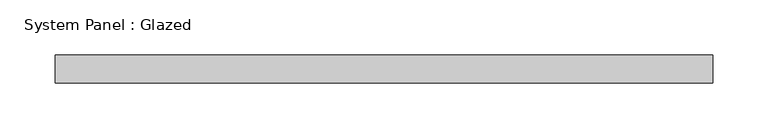
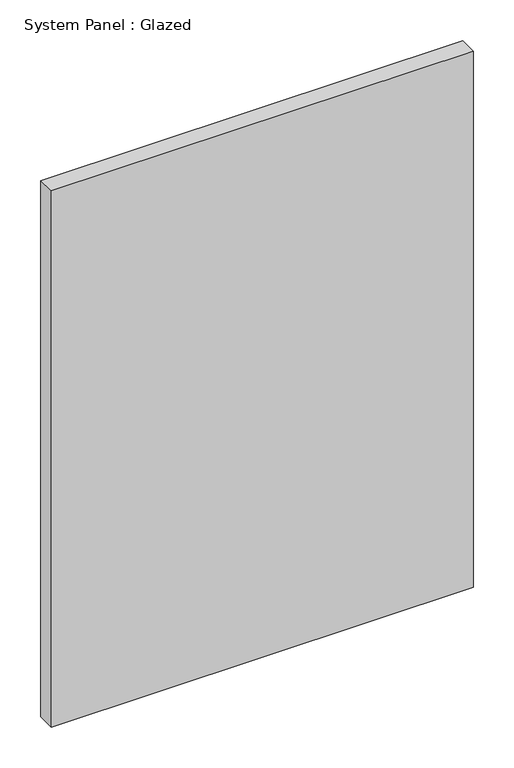
"""IFC4 building model written with IfcOpenShell, lengths in millimetres: plate geometry, System Panel : Glazed."""

from ifc_helpers import new_model, si_unit, origin, origin_with_axes, place, context, project, spatial, polyline, outline, extrude, source, transform, mapped, element, save


def system_panel_glazed_893369a6(model_context):
    return source(origin(), model_context, "Body", "SweptSolid", [
        extrude(outline(polyline([(298.45, 19.05), (-298.45, 19.05), (-298.45, 44.45), (298.45, 44.45), (298.45, 19.05)])), origin_with_axes(), (0.0, 0.0, 1.0), 802.1539078),
    ])


if __name__ == "__main__":
    model = new_model("IFC4")
    model_context = context("Model", 3, world=origin())
    ifc_project = project(units=[si_unit("LENGTHUNIT", "METRE", prefix="MILLI")], contexts=[model_context])
    site = spatial("IfcSite", under=ifc_project)
    building = spatial("IfcBuilding", under=site)
    placement = place(None, origin())
    system_panel_glazed_shape = system_panel_glazed_893369a6(model_context)
    element("IfcPlate", 1, ObjectType="System Panel : Glazed", at=placement, inside=building, context=model_context, shape_type="MappedRepresentation", body=[
        mapped(system_panel_glazed_shape, transform((0.0, 0.0, 0.0), x_axis=(1.0, 0.0, 0.0), y_axis=(0.0, 1.0, 0.0), z_axis=(0.0, 0.0, 1.0))),
    ])
    save(model, "model.ifc")

# Revit data of these elements
# Type "System Panel : Glazed"
#   Construction Type Id = "GSP4R"
#   Analytic Construction = "1/8 in Pilkington single glazing"
#   Visual Light Transmittance = 0.9
#   Solar Heat Gain Coefficient = 0.86
#   Heat Transfer Coefficient (U) = 1.18115 BTU/(h·ft²·°F)
#   Define Thermal Properties by = 1
# Element 1 (IfcPlate, "System Panel : Glazed")
#   Materials on its faces: "Glass"
# Materials
#   "Glass": class "Glass", colour RGB 0 128 192, transparency 0.75, Description = "Soda Lime Glass", Cost = 0
